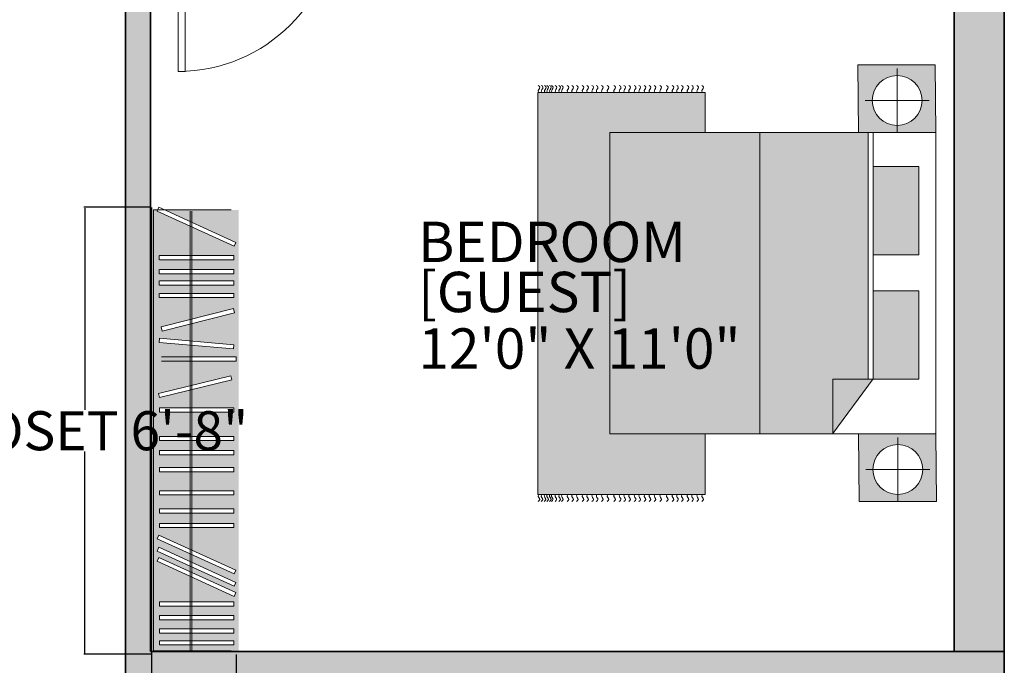
# Model space of a CAD drawing. Units: inches. Extents: x 2167 to 2589, y 1680 to 2489.
# Tile 34 of 38: x 2399 to 2575, y 2027 to 2143. Entities that reach past the tile are written whole.
import ezdxf

# ---------------------------------------------------------------- set-up
doc = ezdxf.new("R2010")
doc.units = ezdxf.units.IN
doc.header["$MEASUREMENT"] = 0
doc.layers.get('0').update_dxf_attribs({"color": 250})
for name, color, linetype, lineweight in [('A-ANNO-DIMS', 2, 'Continuous', 18), ('A-AREA-IDEN', 7, 'Continuous', 18), ('A-DOOR', 4, 'Continuous', 18), ('A-FURN-PATT', 31, 'Continuous', 13), ('A-WALL-PATT', 250, 'Continuous', 13), ('C-PROP', 7, 'Continuous', 35), ('closet', 250, 'Continuous', 18), ('furniture', 34, 'Continuous', 18), ('walls', 7, 'Continuous', 35)]:
    doc.layers.add(name, color=color, linetype=linetype, lineweight=lineweight)
doc.layers.add('A-FURN-FIXD-PATT', color=33, linetype='Continuous', lineweight=13, true_color=0xcd8e5c)
doc.styles.get("Standard").update_dxf_attribs({"font": 'arial.ttf'})
doc.dimstyles.get("Standard").update_dxf_attribs({"dimtxt": 7, "dimasz": 0.18, "dimexe": 0.18, "dimexo": 0.0625, "dimgap": 0.09, "dimtad": 0, "dimtih": 1, "dimtoh": 1, "dimdec": 1, "dimzin": 0, "dimdsep": 46, "dimlunit": 3, "dimtxsty": 'Standard', "dimcen": 0.09, "dimadec": 0, "dimazin": 0, "dimtfac": 1, "dimtdec": 1, "dimtofl": 0, "dimtmove": 0, "dimatfit": 3, "dimfxl": 1, "dimtolj": 1, "dimtzin": 0, "dimarcsym": 0})

# ---------------------------------------------------------------- blocks, each defined once
blk = doc.blocks.new('*U2')
for p, q in [((0, 0), (0, -6)), ((40, 0), (40, -6))]:
    blk.add_line(p, q)
blk.add_lwpolyline([(0, 0), (0, 40), (1.75, 40), (1.75, 0)], close=True)
blk.add_arc((0, 0), 40, 0, 90)
blk = doc.blocks.new('closet')
at = {"layer": 'closet'}
for p, q in [((-0.71, -5.58), (5.59, 8.19)), ((-0.23, 7.39), (-0.23, -6.57)), ((6.27, 7.88), (-0.04, -5.89)), ((5.59, 8.19), (6.27, 7.88)), ((7.92, 7.84), (8.68, 7.84)), ((7.92, 7.84), (7.92, -5.51)), ((8.68, 7.84), (8.68, -5.51)), ((10.44, 7.84), (11.2, 7.84)), ((10.44, 7.84), (10.44, -5.51)), ((11.2, 7.84), (11.2, -5.51)), ((12.45, 7.84), (13.21, 7.84)), ((12.45, 7.84), (12.45, -5.51)), ((13.21, 7.84), (13.21, -5.51)), ((14.71, 7.84), (15.47, 7.84)), ((14.71, 7.84), (14.71, -5.51)), ((15.47, 7.84), (15.47, -5.51)), ((17.44, 7.75), (18.17, 7.93)), ((17.44, 7.75), (20.73, -5.2)), ((18.17, 7.93), (21.46, -5.01)), ((23.92, 7.84), (22.75, -5.46)), ((24.67, 7.78), (23.51, -5.53)), ((23.92, 7.84), (24.67, 7.78)), ((26.09, 8.25), (26.09, -5.1)), ((26.84, 8.25), (26.84, -5.1)), ((29.49, 7.29), (32.64, -5.69)), ((30.22, 7.46), (33.37, -5.51)), ((35.23, 7.84), (35.23, -5.51)), ((35.99, 7.84), (35.99, -5.51)), ((40.33, 7.84), (40.33, -5.51)), ((41.08, 7.84), (41.08, -5.51)), ((42.85, 7.84), (42.85, -5.51)), ((43.61, 7.84), (43.61, -5.51)), ((45.9, 7.84), (45.9, -5.51)), ((46.65, 7.84), (46.65, -5.51)), ((50.07, 7.84), (50.07, -5.51)), ((50.82, 7.84), (50.82, -5.51)), ((53.32, 7.84), (53.32, -5.51)), ((54.08, 7.84), (54.08, -5.51)), ((55.9, 7.84), (55.9, -5.51)), ((56.65, 7.84), (56.65, -5.51)), ((57.99, -5.58), (64.3, 8.19)), ((64.97, 7.88), (58.67, -5.89)), ((60.19, -5.58), (66.49, 8.19)), ((67.17, 7.88), (60.87, -5.89)), ((62, -5.58), (68.3, 8.19)), ((68.98, 7.88), (62.67, -5.89)), ((69.96, 7.84), (69.96, -5.51)), ((70.72, 7.84), (70.72, -5.51)), ((72.43, 7.84), (72.43, -5.51)), ((73.19, 7.84), (73.19, -5.51)), ((74.82, 7.84), (74.82, -5.51)), ((75.57, 7.84), (75.57, -5.51)), ((76.94, 7.84), (76.94, -5.51)), ((77.69, 7.84), (77.69, -5.51)), ((56.23, 0.33), (0, 0.33)), ((56.2, 0), (0, 0)), ((56.2, 0), (78.76, 0)), ((56.23, 0.33), (78.76, 0.33)), ((21.46, -5.01), (20.73, -5.2)), ((-0.04, -5.89), (-0.71, -5.58)), ((23.51, -5.53), (22.75, -5.46)), ((33.37, -5.51), (32.64, -5.69)), ((35.99, -5.51), (35.23, -5.51)), ((41.08, -5.51), (40.33, -5.51)), ((43.61, -5.51), (42.85, -5.51)), ((46.65, -5.51), (45.9, -5.51)), ((50.82, -5.51), (50.07, -5.51)), ((54.08, -5.51), (53.32, -5.51)), ((56.65, -5.51), (55.9, -5.51)), ((58.67, -5.89), (57.99, -5.58)), ((60.87, -5.89), (60.19, -5.58)), ((62.67, -5.89), (62, -5.58)), ((70.72, -5.51), (69.96, -5.51)), ((73.19, -5.51), (72.43, -5.51)), ((75.57, -5.51), (74.82, -5.51)), ((77.69, -5.51), (76.94, -5.51))]:
    blk.add_line(p, q, dxfattribs=at)
blk = doc.blocks.new('rotated closet')
at = {"layer": 'closet'}
for p, q in [((26.32, 0.86), (27.07, 0.86)), ((29.72, -0.11), (30.45, 0.07)), ((35.46, 0.45), (36.22, 0.45)), ((40.56, 0.45), (41.31, 0.45)), ((43.08, 0.45), (43.84, 0.45)), ((46.13, 0.45), (46.88, 0.45)), ((50.3, 0.45), (51.05, 0.45)), ((53.56, 0.45), (54.31, 0.45)), ((56.13, 0.45), (56.88, 0.45)), ((64.53, 0.8), (65.2, 0.49)), ((66.72, 0.8), (67.4, 0.49)), ((68.53, 0.8), (69.21, 0.49)), ((70.19, 0.45), (70.95, 0.45)), ((72.66, 0.45), (73.42, 0.45)), ((75.05, 0.45), (75.81, 0.45)), ((77.17, 0.45), (77.92, 0.45)), ((78.99, 0), (78.99, -13.96)), ((0, -13.96), (78.99, -13.96)), ((8.91, -12.91), (8.15, -12.91)), ((11.43, -12.91), (10.67, -12.91)), ((13.44, -12.91), (12.68, -12.91)), ((15.7, -12.91), (14.94, -12.91)), ((-0.46, -14.27), (79.54, -14.27))]:
    blk.add_line(p, q, dxfattribs=at)
blk.add_blockref('closet', (0.23, -7.39), dxfattribs=at)
blk = doc.blocks.new('CARPET')
at = {"layer": 'furniture'}
for p, q in [((-51.53, -98.11), (-51.53, -55.12)), ((-51.53, -55.12), (-41.27, -55.12)), ((36, -55.12), (51.55, -55.12)), ((51.55, -55.12), (51.55, -98.11)), ((51.55, -98.11), (-51.53, -98.11))]:
    blk.add_line(p, q, dxfattribs=at)
for points, knots in [([(-53.37, -55.99), (-53.22, -55.8), (-52.9, -55.41), (-52.34, -55.8), (-51.89, -56.08), (-51.65, -55.91), (-51.53, -55.83)], [0, 0, 0, 0, 0.653278, 1.290138, 1.740457, 2.114451, 2.114451, 2.114451, 2.114451]), ([(53.37, -55.99), (53.22, -55.8), (52.9, -55.41), (52.34, -55.8), (51.89, -56.08), (51.65, -55.91), (51.53, -55.83)], [0, 0, 0, 0, 0.653278, 1.290138, 1.740457, 2.114451, 2.114451, 2.114451, 2.114451]), ([(-53.37, -57.26), (-53.22, -57.07), (-52.9, -56.67), (-52.34, -57.07), (-51.89, -57.35), (-51.65, -57.17), (-51.53, -57.1)], [0, 0, 0, 0, 0.653278, 1.290138, 1.740457, 2.114451, 2.114451, 2.114451, 2.114451]), ([(53.37, -57.26), (53.22, -57.07), (52.9, -56.67), (52.34, -57.07), (51.89, -57.35), (51.65, -57.17), (51.53, -57.1)], [0, 0, 0, 0, 0.653278, 1.290138, 1.740457, 2.114451, 2.114451, 2.114451, 2.114451]), ([(-53.37, -58.59), (-53.22, -58.4), (-52.9, -58.01), (-52.34, -58.4), (-51.89, -58.68), (-51.65, -58.5), (-51.53, -58.43)], [0, 0, 0, 0, 0.653278, 1.290138, 1.740457, 2.114451, 2.114451, 2.114451, 2.114451]), ([(-53.37, -59.78), (-53.22, -59.58), (-52.9, -59.19), (-52.34, -59.58), (-51.89, -59.86), (-51.65, -59.69), (-51.53, -59.61)], [0, 0, 0, 0, 0.653278, 1.290138, 1.740457, 2.114451, 2.114451, 2.114451, 2.114451]), ([(53.37, -58.59), (53.22, -58.4), (52.9, -58.01), (52.34, -58.4), (51.89, -58.68), (51.65, -58.5), (51.53, -58.43)], [0, 0, 0, 0, 0.653278, 1.290138, 1.740457, 2.114451, 2.114451, 2.114451, 2.114451]), ([(53.37, -59.78), (53.22, -59.58), (52.9, -59.19), (52.34, -59.58), (51.89, -59.86), (51.65, -59.69), (51.53, -59.61)], [0, 0, 0, 0, 0.653278, 1.290138, 1.740457, 2.114451, 2.114451, 2.114451, 2.114451]), ([(-53.37, -61.22), (-53.22, -61.02), (-52.9, -60.63), (-52.34, -61.02), (-51.89, -61.3), (-51.65, -61.13), (-51.53, -61.05)], [0, 0, 0, 0, 0.653278, 1.290138, 1.740457, 2.114451, 2.114451, 2.114451, 2.114451]), ([(-53.37, -62.44), (-53.22, -62.25), (-52.9, -61.86), (-52.34, -62.25), (-51.89, -62.53), (-51.65, -62.36), (-51.53, -62.28)], [0, 0, 0, 0, 0.653278, 1.290138, 1.740457, 2.114451, 2.114451, 2.114451, 2.114451]), ([(53.37, -61.22), (53.22, -61.02), (52.9, -60.63), (52.34, -61.02), (51.89, -61.3), (51.65, -61.13), (51.53, -61.05)], [0, 0, 0, 0, 0.653278, 1.290138, 1.740457, 2.114451, 2.114451, 2.114451, 2.114451]), ([(53.37, -62.44), (53.22, -62.25), (52.9, -61.86), (52.34, -62.25), (51.89, -62.53), (51.65, -62.36), (51.53, -62.28)], [0, 0, 0, 0, 0.653278, 1.290138, 1.740457, 2.114451, 2.114451, 2.114451, 2.114451]), ([(-53.37, -63.63), (-53.22, -63.43), (-52.9, -63.04), (-52.34, -63.43), (-51.89, -63.72), (-51.65, -63.54), (-51.53, -63.46)], [0, 0, 0, 0, 0.653278, 1.290138, 1.740457, 2.114451, 2.114451, 2.114451, 2.114451]), ([(-53.37, -65.07), (-53.22, -64.87), (-52.9, -64.48), (-52.34, -64.87), (-51.89, -65.15), (-51.65, -64.98), (-51.53, -64.9)], [0, 0, 0, 0, 0.653278, 1.290138, 1.740457, 2.114451, 2.114451, 2.114451, 2.114451]), ([(53.37, -63.63), (53.22, -63.43), (52.9, -63.04), (52.34, -63.43), (51.89, -63.72), (51.65, -63.54), (51.53, -63.46)], [0, 0, 0, 0, 0.653278, 1.290138, 1.740457, 2.114451, 2.114451, 2.114451, 2.114451]), ([(53.37, -65.07), (53.22, -64.87), (52.9, -64.48), (52.34, -64.87), (51.89, -65.15), (51.65, -64.98), (51.53, -64.9)], [0, 0, 0, 0, 0.653278, 1.290138, 1.740457, 2.114451, 2.114451, 2.114451, 2.114451]), ([(-53.37, -66.76), (-53.22, -66.56), (-52.9, -66.17), (-52.34, -66.56), (-51.89, -66.84), (-51.65, -66.67), (-51.53, -66.59)], [0, 0, 0, 0, 0.653278, 1.290138, 1.740457, 2.114451, 2.114451, 2.114451, 2.114451]), ([(-53.37, -68.2), (-53.22, -68), (-52.9, -67.61), (-52.34, -68), (-51.89, -68.28), (-51.65, -68.11), (-51.53, -68.03)], [0, 0, 0, 0, 0.653278, 1.290138, 1.740457, 2.114451, 2.114451, 2.114451, 2.114451]), ([(53.37, -66.76), (53.22, -66.56), (52.9, -66.17), (52.34, -66.56), (51.89, -66.84), (51.65, -66.67), (51.53, -66.59)], [0, 0, 0, 0, 0.653278, 1.290138, 1.740457, 2.114451, 2.114451, 2.114451, 2.114451]), ([(53.37, -68.2), (53.22, -68), (52.9, -67.61), (52.34, -68), (51.89, -68.28), (51.65, -68.11), (51.53, -68.03)], [0, 0, 0, 0, 0.653278, 1.290138, 1.740457, 2.114451, 2.114451, 2.114451, 2.114451]), ([(-53.37, -69.53), (-53.22, -69.33), (-52.9, -68.94), (-52.34, -69.33), (-51.89, -69.61), (-51.65, -69.44), (-51.53, -69.36)], [0, 0, 0, 0, 0.653278, 1.290138, 1.740457, 2.114451, 2.114451, 2.114451, 2.114451]), ([(-53.37, -70.79), (-53.22, -70.6), (-52.9, -70.21), (-52.34, -70.6), (-51.89, -70.88), (-51.65, -70.7), (-51.53, -70.63)], [0, 0, 0, 0, 0.653278, 1.290138, 1.740457, 2.114451, 2.114451, 2.114451, 2.114451]), ([(53.37, -69.53), (53.22, -69.33), (52.9, -68.94), (52.34, -69.33), (51.89, -69.61), (51.65, -69.44), (51.53, -69.36)], [0, 0, 0, 0, 0.653278, 1.290138, 1.740457, 2.114451, 2.114451, 2.114451, 2.114451]), ([(53.37, -70.79), (53.22, -70.6), (52.9, -70.21), (52.34, -70.6), (51.89, -70.88), (51.65, -70.7), (51.53, -70.63)], [0, 0, 0, 0, 0.653278, 1.290138, 1.740457, 2.114451, 2.114451, 2.114451, 2.114451]), ([(-53.37, -72.12), (-53.22, -71.93), (-52.9, -71.54), (-52.34, -71.93), (-51.89, -72.21), (-51.65, -72.04), (-51.53, -71.96)], [0, 0, 0, 0, 0.653278, 1.290138, 1.740457, 2.114451, 2.114451, 2.114451, 2.114451]), ([(-53.37, -73.31), (-53.22, -73.11), (-52.9, -72.72), (-52.34, -73.11), (-51.89, -73.4), (-51.65, -73.22), (-51.53, -73.14)], [0, 0, 0, 0, 0.653278, 1.290138, 1.740457, 2.114451, 2.114451, 2.114451, 2.114451]), ([(53.37, -72.12), (53.22, -71.93), (52.9, -71.54), (52.34, -71.93), (51.89, -72.21), (51.65, -72.04), (51.53, -71.96)], [0, 0, 0, 0, 0.653278, 1.290138, 1.740457, 2.114451, 2.114451, 2.114451, 2.114451]), ([(53.37, -73.31), (53.22, -73.11), (52.9, -72.72), (52.34, -73.11), (51.89, -73.4), (51.65, -73.22), (51.53, -73.14)], [0, 0, 0, 0, 0.653278, 1.290138, 1.740457, 2.114451, 2.114451, 2.114451, 2.114451]), ([(-53.37, -74.75), (-53.22, -74.55), (-52.9, -74.16), (-52.34, -74.55), (-51.89, -74.83), (-51.65, -74.66), (-51.53, -74.58)], [0, 0, 0, 0, 0.653278, 1.290138, 1.740457, 2.114451, 2.114451, 2.114451, 2.114451]), ([(-53.37, -75.98), (-53.22, -75.78), (-52.9, -75.39), (-52.34, -75.78), (-51.89, -76.06), (-51.65, -75.89), (-51.53, -75.81)], [0, 0, 0, 0, 0.653278, 1.290138, 1.740457, 2.114451, 2.114451, 2.114451, 2.114451]), ([(53.37, -74.75), (53.22, -74.55), (52.9, -74.16), (52.34, -74.55), (51.89, -74.83), (51.65, -74.66), (51.53, -74.58)], [0, 0, 0, 0, 0.653278, 1.290138, 1.740457, 2.114451, 2.114451, 2.114451, 2.114451]), ([(53.37, -75.98), (53.22, -75.78), (52.9, -75.39), (52.34, -75.78), (51.89, -76.06), (51.65, -75.89), (51.53, -75.81)], [0, 0, 0, 0, 0.653278, 1.290138, 1.740457, 2.114451, 2.114451, 2.114451, 2.114451]), ([(-53.37, -77.16), (-53.22, -76.96), (-52.9, -76.57), (-52.34, -76.96), (-51.89, -77.25), (-51.65, -77.07), (-51.53, -76.99)], [0, 0, 0, 0, 0.653278, 1.290138, 1.740457, 2.114451, 2.114451, 2.114451, 2.114451]), ([(-53.37, -78.6), (-53.22, -78.4), (-52.9, -78.01), (-52.34, -78.4), (-51.89, -78.68), (-51.65, -78.51), (-51.53, -78.43)], [0, 0, 0, 0, 0.653278, 1.290138, 1.740457, 2.114451, 2.114451, 2.114451, 2.114451]), ([(53.37, -77.16), (53.22, -76.96), (52.9, -76.57), (52.34, -76.96), (51.89, -77.25), (51.65, -77.07), (51.53, -76.99)], [0, 0, 0, 0, 0.653278, 1.290138, 1.740457, 2.114451, 2.114451, 2.114451, 2.114451]), ([(53.37, -78.6), (53.22, -78.4), (52.9, -78.01), (52.34, -78.4), (51.89, -78.68), (51.65, -78.51), (51.53, -78.43)], [0, 0, 0, 0, 0.653278, 1.290138, 1.740457, 2.114451, 2.114451, 2.114451, 2.114451]), ([(-53.37, -80.29), (-53.22, -80.09), (-52.9, -79.7), (-52.34, -80.09), (-51.89, -80.37), (-51.65, -80.2), (-51.53, -80.12)], [0, 0, 0, 0, 0.653278, 1.290138, 1.740457, 2.114451, 2.114451, 2.114451, 2.114451]), ([(53.37, -80.29), (53.22, -80.09), (52.9, -79.7), (52.34, -80.09), (51.89, -80.37), (51.65, -80.2), (51.53, -80.12)], [0, 0, 0, 0, 0.653278, 1.290138, 1.740457, 2.114451, 2.114451, 2.114451, 2.114451]), ([(-53.37, -81.73), (-53.22, -81.53), (-52.9, -81.14), (-52.34, -81.53), (-51.89, -81.81), (-51.65, -81.64), (-51.53, -81.56)], [0, 0, 0, 0, 0.653278, 1.290138, 1.740457, 2.114451, 2.114451, 2.114451, 2.114451]), ([(-53.37, -83.06), (-53.22, -82.86), (-52.9, -82.47), (-52.34, -82.86), (-51.89, -83.14), (-51.65, -82.97), (-51.53, -82.89)], [0, 0, 0, 0, 0.653278, 1.290138, 1.740457, 2.114451, 2.114451, 2.114451, 2.114451]), ([(53.37, -81.73), (53.22, -81.53), (52.9, -81.14), (52.34, -81.53), (51.89, -81.81), (51.65, -81.64), (51.53, -81.56)], [0, 0, 0, 0, 0.653278, 1.290138, 1.740457, 2.114451, 2.114451, 2.114451, 2.114451]), ([(53.37, -83.06), (53.22, -82.86), (52.9, -82.47), (52.34, -82.86), (51.89, -83.14), (51.65, -82.97), (51.53, -82.89)], [0, 0, 0, 0, 0.653278, 1.290138, 1.740457, 2.114451, 2.114451, 2.114451, 2.114451]), ([(-53.37, -84.18), (-53.22, -83.99), (-52.9, -83.6), (-52.34, -83.99), (-51.89, -84.27), (-51.65, -84.09), (-51.53, -84.02)], [0, 0, 0, 0, 0.653278, 1.290138, 1.740457, 2.114451, 2.114451, 2.114451, 2.114451]), ([(-53.37, -85.51), (-53.22, -85.32), (-52.9, -84.93), (-52.34, -85.32), (-51.89, -85.6), (-51.65, -85.42), (-51.53, -85.35)], [0, 0, 0, 0, 0.653278, 1.290138, 1.740457, 2.114451, 2.114451, 2.114451, 2.114451]), ([(53.37, -84.18), (53.22, -83.99), (52.9, -83.6), (52.34, -83.99), (51.89, -84.27), (51.65, -84.09), (51.53, -84.02)], [0, 0, 0, 0, 0.653278, 1.290138, 1.740457, 2.114451, 2.114451, 2.114451, 2.114451]), ([(53.37, -85.51), (53.22, -85.32), (52.9, -84.93), (52.34, -85.32), (51.89, -85.6), (51.65, -85.42), (51.53, -85.35)], [0, 0, 0, 0, 0.653278, 1.290138, 1.740457, 2.114451, 2.114451, 2.114451, 2.114451]), ([(-53.37, -86.7), (-53.22, -86.5), (-52.9, -86.11), (-52.34, -86.5), (-51.89, -86.78), (-51.65, -86.61), (-51.53, -86.53)], [0, 0, 0, 0, 0.653278, 1.290138, 1.740457, 2.114451, 2.114451, 2.114451, 2.114451]), ([(-53.37, -88.14), (-53.22, -87.94), (-52.9, -87.55), (-52.34, -87.94), (-51.89, -88.22), (-51.65, -88.05), (-51.53, -87.97)], [0, 0, 0, 0, 0.653278, 1.290138, 1.740457, 2.114451, 2.114451, 2.114451, 2.114451]), ([(53.37, -86.7), (53.22, -86.5), (52.9, -86.11), (52.34, -86.5), (51.89, -86.78), (51.65, -86.61), (51.53, -86.53)], [0, 0, 0, 0, 0.653278, 1.290138, 1.740457, 2.114451, 2.114451, 2.114451, 2.114451]), ([(53.37, -88.14), (53.22, -87.94), (52.9, -87.55), (52.34, -87.94), (51.89, -88.22), (51.65, -88.05), (51.53, -87.97)], [0, 0, 0, 0, 0.653278, 1.290138, 1.740457, 2.114451, 2.114451, 2.114451, 2.114451]), ([(-53.37, -89.36), (-53.22, -89.17), (-52.9, -88.78), (-52.34, -89.17), (-51.89, -89.45), (-51.65, -89.28), (-51.53, -89.2)], [0, 0, 0, 0, 0.653278, 1.290138, 1.740457, 2.114451, 2.114451, 2.114451, 2.114451]), ([(-53.37, -90.55), (-53.22, -90.35), (-52.9, -89.96), (-52.34, -90.35), (-51.89, -90.64), (-51.65, -90.46), (-51.53, -90.38)], [0, 0, 0, 0, 0.653278, 1.290138, 1.740457, 2.114451, 2.114451, 2.114451, 2.114451]), ([(53.37, -89.36), (53.22, -89.17), (52.9, -88.78), (52.34, -89.17), (51.89, -89.45), (51.65, -89.28), (51.53, -89.2)], [0, 0, 0, 0, 0.653278, 1.290138, 1.740457, 2.114451, 2.114451, 2.114451, 2.114451]), ([(53.37, -90.55), (53.22, -90.35), (52.9, -89.96), (52.34, -90.35), (51.9, -90.63), (51.66, -90.47), (51.55, -90.4)], [0, 0, 0, 0, 0.653278, 1.290138, 1.740457, 2.0926, 2.0926, 2.0926, 2.0926]), ([(-53.37, -91.99), (-53.22, -91.79), (-52.9, -91.4), (-52.34, -91.79), (-51.89, -92.07), (-51.65, -91.9), (-51.53, -91.82)], [0, 0, 0, 0, 0.653278, 1.290138, 1.740457, 2.114451, 2.114451, 2.114451, 2.114451]), ([(-53.37, -92.69), (-53.22, -92.48), (-52.9, -92.08), (-52.35, -92.49), (-51.89, -92.77), (-51.65, -92.6), (-51.53, -92.52)], [0, 0, 0, 0, 0.663904, 1.307406, 1.757725, 2.131719, 2.131719, 2.131719, 2.131719]), ([(-53.37, -93.61), (-53.22, -93.42), (-52.9, -93.03), (-52.34, -93.42), (-51.89, -93.7), (-51.65, -93.52), (-51.53, -93.45)], [0, 0, 0, 0, 0.653278, 1.290138, 1.740457, 2.114451, 2.114451, 2.114451, 2.114451]), ([(53.37, -91.99), (53.22, -91.79), (52.9, -91.4), (52.34, -91.79), (51.9, -92.07), (51.66, -91.91), (51.55, -91.83)], [0, 0, 0, 0, 0.653278, 1.290138, 1.740457, 2.0926, 2.0926, 2.0926, 2.0926]), ([(53.37, -92.69), (53.22, -92.49), (52.9, -92.09), (52.34, -92.49), (51.9, -92.77), (51.66, -92.61), (51.55, -92.53)], [0, 0, 0, 0, 0.656792, 1.295826, 1.746145, 2.098292, 2.098292, 2.098292, 2.098292]), ([(53.37, -93.66), (53.22, -93.46), (52.9, -93.07), (52.34, -93.46), (51.9, -93.74), (51.66, -93.58), (51.55, -93.5)], [0, 0, 0, 0, 0.653278, 1.290138, 1.740457, 2.0926, 2.0926, 2.0926, 2.0926]), ([(-53.37, -94.55), (-53.22, -94.35), (-52.9, -93.96), (-52.34, -94.35), (-51.89, -94.63), (-51.65, -94.46), (-51.53, -94.38)], [0, 0, 0, 0, 0.653278, 1.290138, 1.740457, 2.114451, 2.114451, 2.114451, 2.114451]), ([(-53.37, -95.05), (-53.22, -94.85), (-52.9, -94.46), (-52.34, -94.85), (-51.89, -95.14), (-51.65, -94.96), (-51.53, -94.88)], [0, 0, 0, 0, 0.653278, 1.290138, 1.740457, 2.114451, 2.114451, 2.114451, 2.114451]), ([(-53.37, -95.73), (-53.22, -95.54), (-52.9, -95.15), (-52.34, -95.54), (-51.89, -95.82), (-51.65, -95.65), (-51.53, -95.57)], [0, 0, 0, 0, 0.653278, 1.290138, 1.740457, 2.114451, 2.114451, 2.114451, 2.114451]), ([(-53.37, -96.38), (-53.22, -96.18), (-52.9, -95.79), (-52.34, -96.18), (-51.89, -96.47), (-51.65, -96.29), (-51.53, -96.21)], [0, 0, 0, 0, 0.653278, 1.290138, 1.740457, 2.114451, 2.114451, 2.114451, 2.114451]), ([(53.37, -95.78), (53.22, -95.58), (52.9, -95.19), (52.34, -95.58), (51.89, -95.86), (51.65, -95.69), (51.53, -95.61)], [0, 0, 0, 0, 0.653278, 1.290138, 1.740457, 2.114451, 2.114451, 2.114451, 2.114451]), ([(53.37, -96.43), (53.22, -96.23), (52.9, -95.84), (52.34, -96.23), (51.89, -96.51), (51.65, -96.34), (51.53, -96.26)], [0, 0, 0, 0, 0.653278, 1.290138, 1.740457, 2.114451, 2.114451, 2.114451, 2.114451]), ([(53.37, -94.59), (53.22, -94.4), (52.9, -94.01), (52.34, -94.4), (51.9, -94.68), (51.66, -94.51), (51.55, -94.44)], [0, 0, 0, 0, 0.653278, 1.290138, 1.740457, 2.0926, 2.0926, 2.0926, 2.0926]), ([(53.37, -95.1), (53.22, -94.9), (52.9, -94.51), (52.34, -94.9), (51.9, -95.18), (51.66, -95.02), (51.55, -94.94)], [0, 0, 0, 0, 0.653278, 1.290138, 1.740457, 2.0926, 2.0926, 2.0926, 2.0926]), ([(-53.37, -97.17), (-53.22, -96.98), (-52.9, -96.59), (-52.34, -96.98), (-51.89, -97.26), (-51.65, -97.08), (-51.53, -97.01)], [0, 0, 0, 0, 0.653278, 1.290138, 1.740457, 2.114451, 2.114451, 2.114451, 2.114451]), ([(-53.37, -97.99), (-53.22, -97.79), (-52.9, -97.4), (-52.34, -97.79), (-51.89, -98.08), (-51.65, -97.9), (-51.53, -97.82)], [0, 0, 0, 0, 0.653278, 1.290138, 1.740457, 2.114451, 2.114451, 2.114451, 2.114451]), ([(53.37, -97.22), (53.22, -97.02), (52.9, -96.63), (52.34, -97.02), (51.89, -97.3), (51.65, -97.13), (51.53, -97.05)], [0, 0, 0, 0, 0.653278, 1.290138, 1.740457, 2.114451, 2.114451, 2.114451, 2.114451]), ([(53.37, -97.99), (53.22, -97.79), (52.9, -97.4), (52.34, -97.79), (51.89, -98.08), (51.65, -97.9), (51.53, -97.82)], [0, 0, 0, 0, 0.653278, 1.290138, 1.740457, 2.114451, 2.114451, 2.114451, 2.114451])]:
    blk.add_open_spline(points, degree=3, knots=knots, dxfattribs=at)
blk = doc.blocks.new('A$C58D270C6')
at = {"layer": 'furniture'}
for p, q in [((9.09, 124.13), (9.09, 108.87)), ((1.46, 116.5), (16.73, 116.5)), ((14.97, 94.84), (24.62, 107.92)), ((24.62, 94.93), (24.62, 107.92)), ((42.08, 108), (42.08, 36)), ((14.97, 94.93), (24.62, 94.93)), ((14.97, 94.84), (14.97, 36)), ((16.22, 94.93), (16.22, 36)), ((9.25, 36), (9.25, 20.74)), ((1.62, 28.37), (16.88, 28.37))]:
    blk.add_line(p, q, dxfattribs=at)
for points in [[(18.5, 108), (18.34, 124.13), (-0.16, 124.13), (0, 108)], [(0, 108), (77.91, 108), (77.91, 36), (0, 36)], [(4.09, 94.93), (14.97, 94.93), (14.97, 73.83), (4.09, 73.83)], [(4.09, 65.23), (14.97, 65.23), (14.97, 44.13), (4.09, 44.13)], [(18.65, 19.87), (18.5, 36), (0, 36), (0.16, 19.87)]]:
    blk.add_lwpolyline(points, close=True, dxfattribs=at)
for centre in [(9.09, 116.5), (9.25, 28.37)]:
    blk.add_circle(centre, 5.95, dxfattribs=at)
at = {"layer": 'furniture', "xscale": 0.9312884925094044, "yscale": 0.9312884925094044, "zscale": 0.9312884925094044, "rotation": 90}
blk.add_blockref('CARPET', (3.79, 74.47), dxfattribs=at)
blk = doc.blocks.new('*D35')
at = {"layer": 'A-ANNO-DIMS', "color": 0, "lineweight": -2, "transparency": 16777216}
for p, q in [((2422.18, 2109.24), (2410.06, 2109.24)), ((2410.24, 2109.06), (2410.24, 2072.94)), ((2410.24, 2029.39), (2410.24, 2065.51)), ((2422.18, 2029.21), (2410.06, 2029.21))]:
    blk.add_line(p, q, dxfattribs=at)
at = {"layer": 'A-ANNO-DIMS', "color": 0, "transparency": 16777216}
for points in [[(2410.21, 2109.06), (2410.27, 2109.06), (2410.24, 2109.24)], [(2410.21, 2029.39), (2410.27, 2029.39), (2410.24, 2029.21)]]:
    blk.add_solid(points, dxfattribs=at)
at = {"layer": 'Defpoints', "color": 0, "transparency": 16777216}
for p in [(2422.24, 2109.24), (2410.24, 2029.21), (2422.24, 2029.21)]:
    blk.add_point(p, dxfattribs=at)
at = {"layer": 'A-ANNO-DIMS', "color": 0, "transparency": 16777216, "insert": (2410.24, 2069.22), "char_height": 7, "attachment_point": 5}
blk.add_mtext('\\A1;CLOSET 6\'-8"', dxfattribs=at)
blk = doc.blocks.new('*D36')
at = {"layer": 'A-ANNO-DIMS', "color": 0, "lineweight": -2, "transparency": 16777216}
for p, q in [((2422.24, 2029.15), (2422.24, 2017.03)), ((2437.38, 2029.15), (2437.38, 2017.03)), ((2422.42, 2017.21), (2437.2, 2017.21)), ((2437.38, 2017.21), (2437.56, 2017.21))]:
    blk.add_line(p, q, dxfattribs=at)
at = {"layer": 'A-ANNO-DIMS', "color": 0, "transparency": 16777216}
for points in [[(2422.42, 2017.24), (2422.42, 2017.18), (2422.24, 2017.21)], [(2437.2, 2017.24), (2437.2, 2017.18), (2437.38, 2017.21)]]:
    blk.add_solid(points, dxfattribs=at)
at = {"layer": 'Defpoints', "color": 0, "transparency": 16777216}
for p in [(2422.24, 2029.21), (2437.38, 2029.21), (2437.38, 2017.21)]:
    blk.add_point(p, dxfattribs=at)
at = {"layer": 'A-ANNO-DIMS', "color": 0, "transparency": 16777216, "insert": (2446.62, 2017.21), "char_height": 7, "attachment_point": 5}
blk.add_mtext('\\A1;1\'-3"', dxfattribs=at)

msp = doc.modelspace()

# ---------------------------------------------------------------- hatches: boundary and pattern name
at = {"layer": 'A-FURN-FIXD-PATT'}
h = msp.add_hatch(color=256, dxfattribs=at)
h.dxf.hatch_style = 1
h.paths.add_polyline_path([(2423.24, 2045.85), (2423.55, 2046.53), (2429.13, 2043.97), (2429.13, 2044.96), (2423.24, 2047.66), (2423.55, 2048.34), (2429.13, 2045.78), (2429.13, 2047.16), (2423.24, 2049.86), (2423.55, 2050.53), (2429.13, 2047.98), (2429.13, 2051.87), (2423.61, 2051.87), (2423.61, 2052.63), (2429.13, 2052.63), (2429.13, 2054.44), (2423.61, 2054.44), (2423.61, 2055.2), (2429.13, 2055.2), (2429.13, 2057.7), (2423.61, 2057.7), (2423.61, 2058.46), (2429.13, 2058.46), (2429.13, 2061.87), (2423.61, 2061.87), (2423.61, 2062.63), (2429.13, 2062.63), (2429.13, 2064.92), (2423.61, 2064.92), (2423.61, 2065.68), (2429.13, 2065.68), (2429.13, 2067.44), (2423.61, 2067.44), (2423.61, 2068.2), (2429.13, 2068.2), (2429.13, 2072.54), (2423.61, 2072.54), (2423.61, 2073.3), (2429.13, 2073.3), (2429.13, 2076.49), (2423.61, 2075.15), (2423.43, 2075.89), (2429.13, 2077.27), (2429.13, 2084.53), (2423.59, 2085.02), (2423.66, 2085.77), (2429.13, 2085.29), (2429.13, 2088.34), (2424.12, 2087.06), (2423.93, 2087.8), (2429.13, 2089.12), (2429.13, 2093.06), (2423.61, 2093.06), (2423.61, 2093.81), (2429.13, 2093.81), (2429.13, 2095.32), (2423.61, 2095.32), (2423.61, 2096.08), (2429.13, 2096.08), (2429.13, 2097.32), (2423.61, 2097.32), (2423.61, 2098.08), (2429.13, 2098.08), (2429.13, 2099.85), (2423.61, 2099.85), (2423.61, 2100.6), (2429.13, 2100.6), (2429.13, 2105.87), (2423.24, 2108.56), (2423.33, 2108.76), (2422.56, 2108.76), (2422.56, 2029.77), (2429.13, 2029.77), (2429.13, 2030.83), (2423.61, 2030.83), (2423.61, 2031.59), (2429.13, 2031.59), (2429.13, 2032.95), (2423.61, 2032.95), (2423.61, 2033.71), (2429.13, 2033.71), (2429.13, 2035.34), (2423.61, 2035.34), (2423.61, 2036.1), (2429.13, 2036.1), (2429.13, 2037.8), (2423.61, 2037.8), (2423.61, 2038.56), (2429.13, 2038.56), (2429.13, 2043.15)])
h.paths.add_polyline_path([(2429.46, 2043), (2429.46, 2038.56), (2436.97, 2038.56), (2436.97, 2037.8), (2429.46, 2037.8), (2429.46, 2036.1), (2436.97, 2036.1), (2436.97, 2035.34), (2429.46, 2035.34), (2429.46, 2033.71), (2436.97, 2033.71), (2436.97, 2032.95), (2429.46, 2032.95), (2429.46, 2031.59), (2436.97, 2031.59), (2436.97, 2030.83), (2429.46, 2030.83), (2429.46, 2029.77), (2436.52, 2029.77), (2437.37, 2029.77), (2437.81, 2029.77), (2437.81, 2108.76), (2424.6, 2108.76), (2437.32, 2102.93), (2437.01, 2102.26), (2429.46, 2105.71), (2429.46, 2100.6), (2436.97, 2100.6), (2436.97, 2099.85), (2429.46, 2099.85), (2429.46, 2098.08), (2436.97, 2098.08), (2436.97, 2097.32), (2429.46, 2097.32), (2429.46, 2096.08), (2436.97, 2096.08), (2436.97, 2095.32), (2429.46, 2095.32), (2429.46, 2093.81), (2436.97, 2093.81), (2436.97, 2093.06), (2429.46, 2093.06), (2429.46, 2089.2), (2436.87, 2091.09), (2437.06, 2090.36), (2429.46, 2088.42), (2429.46, 2085.26), (2436.97, 2084.61), (2436.9, 2083.85), (2429.46, 2084.5), (2429.46, 2082.44), (2437.38, 2082.44), (2437.38, 2081.68), (2429.46, 2081.68), (2429.46, 2077.35), (2436.41, 2079.04), (2436.59, 2078.3), (2429.46, 2076.57), (2429.46, 2073.3), (2436.97, 2073.3), (2436.97, 2072.54), (2429.46, 2072.54), (2429.46, 2068.2), (2436.97, 2068.2), (2436.97, 2067.44), (2429.46, 2067.44), (2429.46, 2065.68), (2436.97, 2065.68), (2436.97, 2064.92), (2429.46, 2064.92), (2429.46, 2062.63), (2436.97, 2062.63), (2436.97, 2061.87), (2429.46, 2061.87), (2429.46, 2058.46), (2436.97, 2058.46), (2436.97, 2057.7), (2429.46, 2057.7), (2429.46, 2055.2), (2436.97, 2055.2), (2436.97, 2054.44), (2429.46, 2054.44), (2429.46, 2052.63), (2436.97, 2052.63), (2436.97, 2051.87), (2429.46, 2051.87), (2429.46, 2047.82), (2437.32, 2044.23), (2437.01, 2043.55), (2429.46, 2047.01), (2429.46, 2045.63), (2437.32, 2042.03), (2437.01, 2041.36), (2429.46, 2044.81), (2429.46, 2043.82), (2437.32, 2040.22), (2437.01, 2039.55)])
at = {"layer": 'A-FURN-PATT'}
h = msp.add_hatch(color=256, dxfattribs=at)
h.dxf.hatch_style = 1
h.paths.add_polyline_path([(2551.38, 2128.38, -1), (2560.32, 2128.38, -0.414214), (2555.85, 2123.92), (2555.85, 2122.66), (2562.79, 2122.66), (2562.67, 2134.76), (2548.8, 2134.76), (2548.91, 2122.66), (2555.85, 2122.66), (2555.85, 2123.92, -0.414214)])
h.paths.add_polyline_path([(2560.43, 2062.28, -0.414214), (2555.97, 2057.82), (2555.97, 2056.56), (2562.9, 2056.56), (2562.79, 2068.66), (2548.91, 2068.66), (2549.03, 2056.56), (2555.97, 2056.56), (2555.97, 2057.82, -0.414214), (2551.5, 2062.28, -1)])
h.paths.add_polyline_path([(2551.51, 2078.46), (2544.32, 2078.46), (2544.32, 2068.72)])
h = msp.add_hatch(color=256, dxfattribs=at)
h.dxf.hatch_style = 1
h.paths.add_polyline_path([(2504.36, 2122.66), (2521.44, 2122.66), (2521.44, 2129.8), (2491.42, 2129.8), (2491.42, 2057.8), (2521.44, 2057.8), (2521.44, 2068.66), (2504.36, 2068.66)])
h.paths.add_polyline_path([(2531.23, 2122.66), (2504.36, 2122.66), (2504.36, 2068.66), (2531.23, 2068.66)])
h = msp.add_hatch(color=256, dxfattribs=at)
h.dxf.hatch_style = 1
h.paths.add_polyline_path([(2550.62, 2122.66), (2531.23, 2122.66), (2531.23, 2068.66), (2544.28, 2068.66), (2544.32, 2068.72), (2544.32, 2078.46), (2550.62, 2078.46)])
h = msp.add_hatch(color=256, dxfattribs=at)
h.dxf.hatch_style = 1
h.paths.add_polyline_path([(2559.72, 2116.56), (2551.56, 2116.56), (2551.56, 2100.74), (2559.72, 2100.74)])
h.paths.add_polyline_path([(2559.72, 2094.28), (2551.56, 2094.28), (2551.56, 2078.46), (2559.72, 2078.46)])
at = {"layer": 'A-WALL-PATT'}
h = msp.add_hatch(color=256, dxfattribs=at)
h.dxf.hatch_style = 1
h.paths.add_polyline_path([(2575.05, 2029.69), (2422.05, 2029.69), (2422.05, 2161.69), (2427.02, 2161.69), (2427.02, 2161.94), (2427.02, 2166.19), (2417.55, 2166.19), (2417.55, 2025.19), (2575.05, 2025.19)])
h.paths.add_polyline_path([(2575.05, 2166.19), (2503.01, 2166.19), (2503.01, 2161.69), (2575.05, 2161.69)], flags=17)
h.paths.add_polyline_path([(2575.05, 2161.69), (2566.05, 2161.69), (2566.05, 2029.69), (2575.05, 2029.69)], flags=17)
h.paths.add_polyline_path([(2575.05, 2025.19), (2566.05, 2025.19), (2566.05, 1869.19), (2575.05, 1869.19)])
h.paths.add_polyline_path([(2575.05, 1869.19), (2566.05, 1869.19), (2447.7, 1869.19, -0.014764), (2447.74, 1867.92), (2447.74, 1864.69), (2575.05, 1864.69)])
h.paths.add_polyline_path([(2530.05, 1864.69), (2525.55, 1864.69), (2525.55, 1816.69), (2452.05, 1816.69), (2452.05, 1812.19), (2530.05, 1812.19)])
h.paths.add_polyline_path([(2455.04, 1830.65), (2452.05, 1830.65), (2452.05, 1816.69), (2455.04, 1816.69)], flags=17)
h.paths.add_polyline_path([(2575.05, 1864.69), (2566.05, 1864.69), (2566.05, 1788.19), (2456.1, 1788.19), (2456.1, 1783.94, -0.042065), (2455.7, 1779.19), (2527.68, 1779.19), (2527.68, 1687.69), (2532.18, 1687.69), (2532.18, 1779.19), (2575.05, 1779.19)])
h.paths.add_polyline_path([(2421.87, 1696.69), (2416.11, 1696.69), (2416.11, 1687.69), (2421.87, 1687.69)])
h.paths.add_polyline_path([(2375.61, 1696.69), (2369.84, 1696.69), (2369.84, 1687.69), (2375.61, 1687.69)])
h.paths.add_polyline_path([(2425.05, 2245.69), (2420.55, 2245.69), (2420.55, 2226.19), (2432.29, 2226.19), (2432.29, 2229.42), (2432.29, 2230.69), (2425.05, 2230.69)])
h.paths.add_polyline_path([(2224.05, 2151.19), (2318.55, 2151.19), (2318.55, 2177.3), (2314.78, 2177.3, -0.007324), (2314.05, 2177.32), (2314.05, 2155.69), (2224.05, 2155.69), (2224.05, 2157.46), (2215.05, 2157.46), (2215.05, 2103.59), (2218.97, 2103.59), (2224.05, 2103.59)])

# ---------------------------------------------------------------- linework, layer by layer
at = {"layer": 'C-PROP'}
msp.add_line((2575.05, 2407.69), (2575.05, 1687.69), dxfattribs=at)
at = {"layer": 'closet'}
for p, q in [((2422.24, 2029.21), (2422.24, 2109.21)), ((2422.56, 2108.76), (2422.56, 2029.77)), ((2422.56, 2108.76), (2436.52, 2108.76)), ((2437.45, 2029.69), (2422.24, 2029.69)), ((2422.24, 2029.69), (2422.24, 2029.21)), ((2422.56, 2029.77), (2436.52, 2029.77))]:
    msp.add_line(p, q, dxfattribs=at)
at = {"layer": 'walls'}
for p, q in [((2417.55, 2166.19), (2417.55, 2025.19)), ((2422.05, 2161.69), (2422.05, 2029.69)), ((2566.05, 2161.69), (2566.05, 2029.69)), ((2422.05, 2029.69), (2575.05, 2029.69))]:
    msp.add_line(p, q, dxfattribs=at)

# ---------------------------------------------------------------- block references
at = {"layer": 'A-DOOR', "xscale": -0.7089553820317277, "yscale": 0.7089553820317277, "zscale": 0.7089553820317277, "rotation": 180}
msp.add_blockref('*U2', (2427.02, 2161.94), dxfattribs=at)
at = {"layer": 'closet', "rotation": 269.9999999992008}
msp.add_blockref('rotated closet', (2436.52, 2108.76), dxfattribs=at)
at = {"layer": 'furniture', "xscale": 0.7500000390647866, "yscale": 0.7500000390647866, "zscale": 0.7500000390647866, "rotation": 180}
msp.add_blockref('A$C58D270C6', (2562.79, 2149.66), dxfattribs=at)

# ---------------------------------------------------------------- texts
at = {"layer": 'A-AREA-IDEN'}
for s, height, p in [('BEDROOM', 7.227, (2470.01, 2099.43)), ('[GUEST]', 7.227, (2470.01, 2090.46)), ('12\'0" X 11\'0"', 7.2272, (2470.05, 2080.33))]:
    msp.add_text(s, height=height, dxfattribs=at).set_placement(p)

# ---------------------------------------------------------------- dimensions: what is measured, and where the dimension line sits
at = {"layer": 'A-ANNO-DIMS'}
dim = msp.add_linear_dim(base=(2410.24, 2029.21), p1=(2422.24, 2109.24), p2=(2422.24, 2029.21), angle=270, text='CLOSET <>', dimstyle='Standard', override={"dimdec": 1, "dimlfac": 1, "dimrnd": 0, "dimzin": 1, "dimdsep": 46, "dimlunit": 4, "dimfrac": 2}, dxfattribs=at)
dim.commit()
dim.dimension.update_dxf_attribs({"geometry": '*D35', "text_midpoint": (2410.24, 2069.22)})
dim = msp.add_linear_dim(base=(2437.38, 2017.21), p1=(2422.24, 2029.21), p2=(2437.38, 2029.21), dimstyle='Standard', override={"dimdec": 1, "dimlfac": 1, "dimrnd": 0, "dimzin": 1, "dimdsep": 46, "dimlunit": 4, "dimfrac": 2}, dxfattribs=at)
dim.commit()
dim.dimension.update_dxf_attribs({"geometry": '*D36', "text_midpoint": (2446.62, 2017.21)})

doc.saveas('drawing.dxf')
